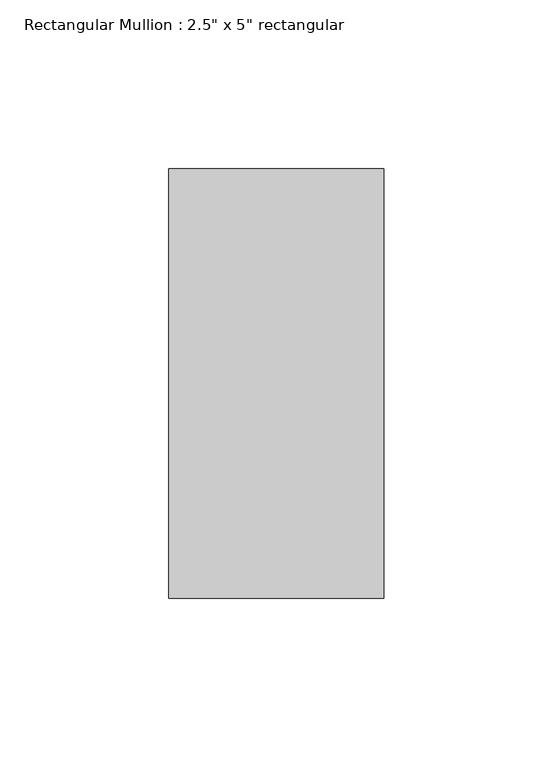
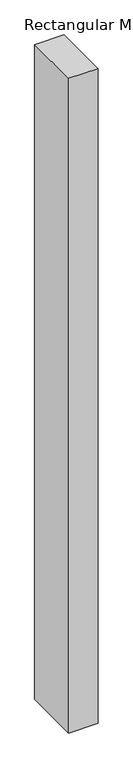
"""IFC4 building model written with IfcOpenShell, lengths in millimetres: member geometry."""

from ifc_helpers import new_model, si_unit, frame, origin, place, context, project, spatial, polyline, outline, extrude, source, transform, mapped, element, save


def member_ecafcbb3(model_context):
    return source(origin(), model_context, "Body", "SweptSolid", [
        extrude(outline(polyline([(0.0, 63.5), (0.0, -63.5), (-63.5, -63.5), (-63.5, 63.5), (0.0, 63.5)])), frame((0.0, 0.0, -1492.25), z_axis=(0.0, 0.0, 1.0), x_axis=(1.0, 0.0, 0.0)), (0.0, 0.0, 1.0), 1492.25),
    ])


if __name__ == "__main__":
    model = new_model("IFC4")
    model_context = context("Model", 3, world=origin())
    ifc_project = project(units=[si_unit("LENGTHUNIT", "METRE", prefix="MILLI")], contexts=[model_context])
    site = spatial("IfcSite", under=ifc_project)
    building = spatial("IfcBuilding", under=site)
    placement = place(None, origin())
    member_shape = member_ecafcbb3(model_context)
    element("IfcMember", 1, ObjectType="Rectangular Mullion : 2.5\" x 5\" rectangular", at=placement, inside=building, context=model_context, shape_type="MappedRepresentation", body=[
        mapped(member_shape, transform((0.0, 0.0, 0.0), x_axis=(1.0, 0.0, 0.0), y_axis=(0.0, 1.0, 0.0), z_axis=(0.0, 0.0, 1.0))),
    ])
    save(model, "model.ifc")

# Revit data of these elements
# Type "Rectangular Mullion : 2.5\" x 5\" rectangular"
#   built-in parameter 1007304 = 0.416667 (stored number, unit not read)
#   built-in parameter 1007301 = 0.104167 (stored number, unit not read)
#   built-in parameter 1007300 = 0.104167 (stored number, unit not read)
# Element 1 (IfcMember, "Rectangular Mullion : 2.5\" x 5\" rectangular")
#   Materials on its faces: "Aluminum"
# Materials
#   "Aluminum": class "Metal", colour RGB 247 247 247, transparency 0, Description = "Aluminum 6061", Cost = 0
